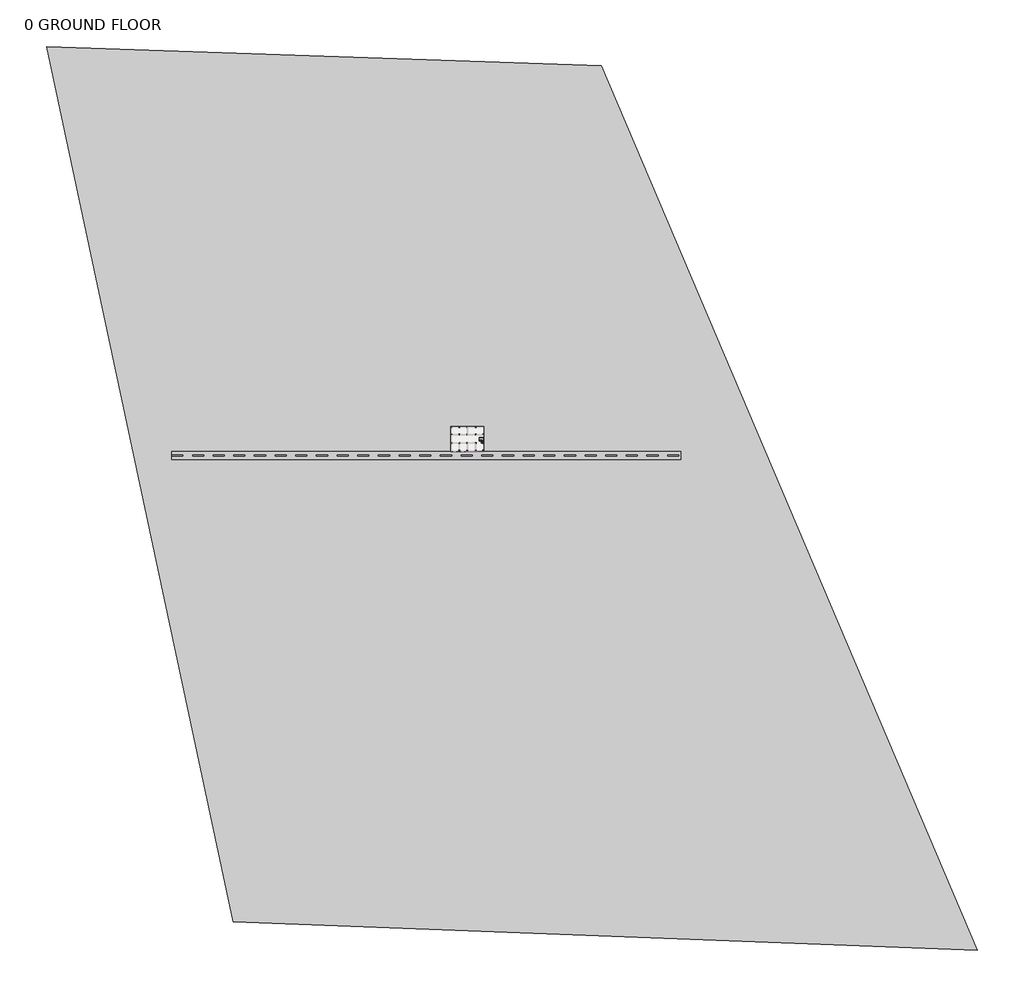
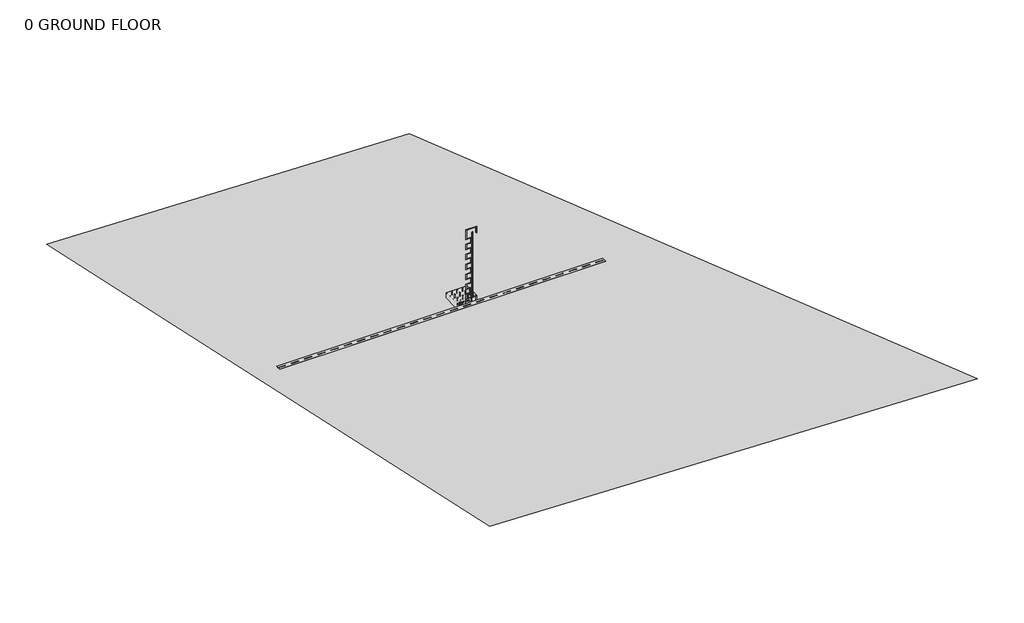
# One storey, part 2 of 2: 18 columns, 13 proxies, 4 members, 3 dampers, 2 cable carrier fittings, 1 stair flight.
"""IFC4 building model written with IfcOpenShell, lengths in millimetres."""

from ifc_helpers import new_model, si_unit, frame, origin, place, context, project, spatial, polyline, outline, extrude, faceted_brep, triangles, transform, mapped, element, save
from components import muntin_pattern_2x2_muntin_pattern_2x2_b3fe6957, muntin_pattern_2x2_muntin_pattern_2x2_3e0ecaf2, trim_window_exterior_flat_with_sill_41619996, trim_window_interior_flat_picture_frame_51c85655, conduit_fittings_1_conduit_fittings_1_d54f14cf, conduit_fittings_2_conduit_fittings_2_af195c82, duct_accessories_13_duct_accessories_1_4da7b8f5, duct_accessories_15_duct_accessories_15_503ec04a, duct_accessories_16_duct_accessories_15_820109d7, stair_flight_2b9b7e9b

model = new_model("IFC4")

# Units and contexts
model_context = context("Model", 3, world=origin())
ifc_project = project(units=[si_unit("LENGTHUNIT", "METRE", prefix="MILLI")], contexts=[model_context])

# Site, building, storey
site = spatial("IfcSite", under=ifc_project)
building = spatial("IfcBuilding", under=site)
storey = spatial("IfcBuildingStorey", under=building, Name="0 GROUND FLOOR", Elevation=0.0)

# Proxies
placement = place(None, origin())
element("IfcBuildingElementProxy", 1, Name="Building Element Proxy", at=placement, inside=storey, context=model_context, shape_type="Tessellation", body=[
    triangles([(-164952.4245117, 149002.5980713, 0.0), (39631.450708, 141833.0729004, 0.0), (178424.9416992, -184532.3270508, 0.0), (-96169.5159668, -174046.6042969, 0.0)], [[1, 4, 2], [3, 2, 4]], closed=False),
])
muntin_pattern_2x2_muntin_pattern_2x2_shape = muntin_pattern_2x2_muntin_pattern_2x2_b3fe6957(model_context)
element("IfcBuildingElementProxy", 2, Name="Muntin Pattern_2x2 : Muntin Pattern_2x2", ObjectType="Muntin Pattern_2x2 : Muntin Pattern_2x2", at=placement, inside=storey, context=model_context, shape_type="MappedRepresentation", body=[
    mapped(muntin_pattern_2x2_muntin_pattern_2x2_shape, transform((-14441.409625, -253.8184478, 984.25), x_axis=(1.0, 0.0, 0.0), y_axis=(0.0, 1.0, 0.0), z_axis=(0.0, 0.0, 1.0))),
])
element("IfcBuildingElementProxy", 3, Name="Muntin Pattern_2x2 : Muntin Pattern_2x2", ObjectType="Muntin Pattern_2x2 : Muntin Pattern_2x2", at=placement, inside=storey, context=model_context, shape_type="MappedRepresentation", body=[
    mapped(muntin_pattern_2x2_muntin_pattern_2x2_shape, transform((-11393.409625, -253.8184478, 984.25), x_axis=(1.0, 0.0, 0.0), y_axis=(0.0, 1.0, 0.0), z_axis=(0.0, 0.0, 1.0))),
])
element("IfcBuildingElementProxy", 4, Name="Muntin Pattern_2x2 : Muntin Pattern_2x2", ObjectType="Muntin Pattern_2x2 : Muntin Pattern_2x2", at=placement, inside=storey, context=model_context, shape_type="MappedRepresentation", body=[
    mapped(muntin_pattern_2x2_muntin_pattern_2x2_shape, transform((-8650.209625, -253.8184478, 984.25), x_axis=(1.0, 0.0, 0.0), y_axis=(0.0, 1.0, 0.0), z_axis=(0.0, 0.0, 1.0))),
])
muntin_pattern_2x2_muntin_pattern_2x2_2_shape = muntin_pattern_2x2_muntin_pattern_2x2_3e0ecaf2(model_context)
element("IfcBuildingElementProxy", 5, Name="Muntin Pattern_2x2 : Muntin Pattern_2x2", ObjectType="Muntin Pattern_2x2 : Muntin Pattern_2x2", at=placement, inside=storey, context=model_context, shape_type="MappedRepresentation", body=[
    mapped(muntin_pattern_2x2_muntin_pattern_2x2_2_shape, transform((-14012.784625, -253.8184478, 984.25), x_axis=(-1.0, 0.0, 0.0), y_axis=(0.0, -1.0, 0.0), z_axis=(0.0, 0.0, 1.0))),
])
element("IfcBuildingElementProxy", 6, Name="Muntin Pattern_2x2 : Muntin Pattern_2x2", ObjectType="Muntin Pattern_2x2 : Muntin Pattern_2x2", at=placement, inside=storey, context=model_context, shape_type="MappedRepresentation", body=[
    mapped(muntin_pattern_2x2_muntin_pattern_2x2_2_shape, transform((-10964.784625, -253.8184478, 984.25), x_axis=(-1.0, 0.0, 0.0), y_axis=(0.0, -1.0, 0.0), z_axis=(0.0, 0.0, 1.0))),
])
element("IfcBuildingElementProxy", 7, Name="Muntin Pattern_2x2 : Muntin Pattern_2x2", ObjectType="Muntin Pattern_2x2 : Muntin Pattern_2x2", at=placement, inside=storey, context=model_context, shape_type="MappedRepresentation", body=[
    mapped(muntin_pattern_2x2_muntin_pattern_2x2_2_shape, transform((-8221.584625, -253.8184478, 984.25), x_axis=(-1.0, 0.0, 0.0), y_axis=(0.0, -1.0, 0.0), z_axis=(0.0, 0.0, 1.0))),
])
trim_window_exterior_flat_with_sill_shape = trim_window_exterior_flat_with_sill_41619996(model_context)
element("IfcBuildingElementProxy", 8, Name="Trim-Window-Exterior-Flat : with Sill", ObjectType="Trim-Window-Exterior-Flat : with Sill", at=placement, inside=storey, context=model_context, shape_type="MappedRepresentation", body=[
    mapped(trim_window_exterior_flat_with_sill_shape, transform((-14227.097125, -244.2934478, 1828.8), x_axis=(-1.0, 0.0, 0.0), y_axis=(0.0, 0.0, 1.0), z_axis=(0.0, 1.0, 0.0))),
])
element("IfcBuildingElementProxy", 9, Name="Trim-Window-Exterior-Flat : with Sill", ObjectType="Trim-Window-Exterior-Flat : with Sill", at=placement, inside=storey, context=model_context, shape_type="MappedRepresentation", body=[
    mapped(trim_window_exterior_flat_with_sill_shape, transform((-11179.097125, -244.2934478, 1828.8), x_axis=(-1.0, 0.0, 0.0), y_axis=(0.0, 0.0, 1.0), z_axis=(0.0, 1.0, 0.0))),
])
element("IfcBuildingElementProxy", 10, Name="Trim-Window-Exterior-Flat : with Sill", ObjectType="Trim-Window-Exterior-Flat : with Sill", at=placement, inside=storey, context=model_context, shape_type="MappedRepresentation", body=[
    mapped(trim_window_exterior_flat_with_sill_shape, transform((-8435.897125, -244.2934478, 1828.8), x_axis=(-1.0, 0.0, 0.0), y_axis=(0.0, 0.0, 1.0), z_axis=(0.0, 1.0, 0.0))),
])
trim_window_interior_flat_picture_frame_shape = trim_window_interior_flat_picture_frame_51c85655(model_context)
element("IfcBuildingElementProxy", 11, Name="Trim-Window-Interior-Flat : Picture Frame", ObjectType="Trim-Window-Interior-Flat : Picture Frame", at=placement, inside=storey, context=model_context, shape_type="MappedRepresentation", body=[
    mapped(trim_window_interior_flat_picture_frame_shape, transform((-14227.097125, -371.2934478, 1828.8), x_axis=(1.0, 0.0, 0.0), y_axis=(0.0, 0.0, 1.0), z_axis=(0.0, -1.0, 0.0))),
])
element("IfcBuildingElementProxy", 12, Name="Trim-Window-Interior-Flat : Picture Frame", ObjectType="Trim-Window-Interior-Flat : Picture Frame", at=placement, inside=storey, context=model_context, shape_type="MappedRepresentation", body=[
    mapped(trim_window_interior_flat_picture_frame_shape, transform((-11179.097125, -371.2934478, 1828.8), x_axis=(1.0, 0.0, 0.0), y_axis=(0.0, 0.0, 1.0), z_axis=(0.0, -1.0, 0.0))),
])
element("IfcBuildingElementProxy", 13, Name="Trim-Window-Interior-Flat : Picture Frame", ObjectType="Trim-Window-Interior-Flat : Picture Frame", at=placement, inside=storey, context=model_context, shape_type="MappedRepresentation", body=[
    mapped(trim_window_interior_flat_picture_frame_shape, transform((-8435.897125, -371.2934478, 1828.8), x_axis=(1.0, 0.0, 0.0), y_axis=(0.0, 0.0, 1.0), z_axis=(0.0, -1.0, 0.0))),
])

# Cable carrier fittings
conduit_fittings_1_conduit_fittings_1_shape = conduit_fittings_1_conduit_fittings_1_d54f14cf(model_context)
element("IfcCableCarrierFitting", 14, ObjectType="Conduit Fittings 1 : Conduit Fittings 1", at=placement, inside=storey, context=model_context, shape_type="MappedRepresentation", body=[
    mapped(conduit_fittings_1_conduit_fittings_1_shape, transform((0.0, 0.0, 0.0), x_axis=(1.0, 0.0, 0.0), y_axis=(0.0, 1.0, 0.0), z_axis=(0.0, 0.0, 1.0))),
])
conduit_fittings_2_conduit_fittings_2_shape = conduit_fittings_2_conduit_fittings_2_af195c82(model_context)
element("IfcCableCarrierFitting", 15, ObjectType="Conduit Fittings 2 : Conduit Fittings 2", at=placement, inside=storey, context=model_context, shape_type="MappedRepresentation", body=[
    mapped(conduit_fittings_2_conduit_fittings_2_shape, transform((0.0, 0.0, 0.0), x_axis=(1.0, 0.0, 0.0), y_axis=(0.0, 1.0, 0.0), z_axis=(0.0, 0.0, 1.0))),
])

# Columns
element("IfcColumn", 16, ObjectType="column family : column family", at=placement, inside=storey, context=model_context, shape_type="SweptSolid", body=[
    extrude(outline(polyline([(-15433.597125, 8645.7065522), (-15433.597125, 8391.7065522), (-15687.597125, 8391.7065522), (-15687.597125, 8645.7065522), (-15433.597125, 8645.7065522)])), frame((0.0, 0.0, 5.0), z_axis=(0.0, 0.0, 1.0), x_axis=(1.0, 0.0, 0.0)), (0.0, 0.0, 1.0), 3038.0),
])
element("IfcColumn", 17, ObjectType="column family : column family", at=placement, inside=storey, context=model_context, shape_type="SweptSolid", body=[
    extrude(outline(polyline([(-12576.097125, 5915.2065522), (-12576.097125, 5534.2065522), (-12957.097125, 5534.2065522), (-12957.097125, 5915.2065522), (-12576.097125, 5915.2065522)])), frame((0.0, 0.0, 5.0), z_axis=(0.0, 0.0, 1.0), x_axis=(1.0, 0.0, 0.0)), (0.0, 0.0, 1.0), 3038.0),
])
element("IfcColumn", 18, ObjectType="column family : column family", at=placement, inside=storey, context=model_context, shape_type="Brep", body=[
    faceted_brep([(-9655.097125, 5915.2065522, 5.0), (-9528.097125, 5915.2065522, 5.0), (-9528.097125, 5788.2065522, 5.0), (-9655.097125, 5788.2065522, 5.0), (-9528.097125, 5915.2065522, 3043.0), (-9655.097125, 5915.2065522, 3043.0), (-9655.097125, 5788.2065522, 3043.0), (-9528.097125, 5788.2065522, 3043.0)], [[[0, 1, 2, 3]], [[4, 5, 6, 7]], [[0, 3, 6, 5]], [[4, 1, 0, 5]], [[3, 2, 7, 6]], [[1, 4, 7, 2]]]),
    faceted_brep([(-9528.097125, 5534.2065522, 3043.0), (-9528.097125, 5534.2065522, 5.0), (-9528.097125, 5661.2065522, 5.0), (-9528.097125, 5661.2065522, 3043.0), (-9909.097125, 5534.2065522, 5.0), (-9909.097125, 5534.2065522, 3043.0), (-9909.097125, 5915.2065522, 5.0), (-9909.097125, 5661.2065522, 3043.0), (-9909.097125, 5661.2065522, 2133.6), (-9909.097125, 5788.2065522, 2133.6), (-9909.097125, 5788.2065522, 3043.0), (-9909.097125, 5915.2065522, 3043.0), (-9782.097125, 5915.2065522, 3043.0), (-9782.097125, 5915.2065522, 5.0), (-9782.097125, 5788.2065522, 5.0), (-9782.097125, 5788.2065522, 3043.0), (-9782.097125, 5788.2065522, 2133.6), (-9718.597125, 5788.2065522, 5.0), (-9718.597125, 5788.2065522, 2133.6), (-9718.597125, 5661.2065522, 5.0), (-9718.597125, 5661.2065522, 2133.6)], [[[0, 1, 2, 3]], [[4, 1, 0, 5]], [[6, 4, 5, 7, 8, 9, 10, 11]], [[6, 11, 12, 13]], [[14, 13, 12, 15, 16]], [[17, 14, 16, 18]], [[19, 20, 8, 7, 3, 2]], [[1, 4, 6, 13, 14, 17, 19, 2]], [[5, 0, 3, 7]], [[12, 11, 10, 15]], [[9, 16, 15, 10]], [[18, 20, 19, 17]], [[20, 18, 16, 9, 8]]]),
])
element("IfcColumn", 19, ObjectType="column family : column family", at=placement, inside=storey, context=model_context, shape_type="Brep", body=[
    faceted_brep([(-6480.097125, 5534.2065522, 5.0), (-6861.097125, 5534.2065522, 5.0), (-6861.097125, 5915.2065522, 5.0), (-6480.097125, 5915.2065522, 5.0), (-6480.097125, 5788.2065522, 5.0), (-6670.597125, 5788.2065522, 5.0), (-6670.597125, 5661.2065522, 5.0), (-6480.097125, 5661.2065522, 5.0), (-6480.097125, 5534.2065522, 3043.0), (-6480.097125, 5661.2065522, 3043.0), (-6861.097125, 5534.2065522, 3043.0), (-6861.097125, 5661.2065522, 3043.0), (-6861.097125, 5661.2065522, 2133.6), (-6861.097125, 5788.2065522, 2133.6), (-6861.097125, 5788.2065522, 3043.0), (-6861.097125, 5915.2065522, 3043.0), (-6480.097125, 5915.2065522, 3043.0), (-6670.597125, 5661.2065522, 2133.6), (-6670.597125, 5788.2065522, 2133.6), (-6480.097125, 5788.2065522, 3043.0)], [[[0, 1, 2, 3, 4, 5, 6, 7]], [[8, 0, 7, 9]], [[1, 0, 8, 10]], [[2, 1, 10, 11, 12, 13, 14, 15]], [[3, 2, 15, 16]], [[10, 8, 9, 11]], [[6, 17, 12, 11, 9, 7]], [[13, 18, 5, 4, 19, 14]], [[3, 16, 19, 4]], [[16, 15, 14, 19]], [[18, 17, 6, 5]], [[17, 18, 13, 12]]]),
])
element("IfcColumn", 20, ObjectType="column family : column family", at=placement, inside=storey, context=model_context, shape_type="Brep", body=[
    faceted_brep([(-6480.097125, 2867.2065522, 5.0), (-6480.097125, 2486.2065522, 5.0), (-6645.197125, 2486.2065522, 5.0), (-6645.197125, 2740.2065522, 5.0), (-6708.697125, 2740.2065522, 5.0), (-6708.697125, 2613.2065522, 5.0), (-6772.197125, 2613.2065522, 5.0), (-6772.197125, 2486.2065522, 5.0), (-6861.097125, 2486.2065522, 5.0), (-6861.097125, 2867.2065522, 5.0), (-6480.097125, 2867.2065522, 3043.0), (-6480.097125, 2486.2065522, 3043.0), (-6861.097125, 2486.2065522, 3043.0), (-6772.197125, 2486.2065522, 3043.0), (-6861.097125, 2613.2065522, 3043.0), (-6861.097125, 2613.2065522, 2133.6), (-6861.097125, 2740.2065522, 2133.6), (-6861.097125, 2740.2065522, 3043.0), (-6861.097125, 2867.2065522, 3043.0), (-6772.197125, 2740.2065522, 3043.0), (-6645.197125, 2740.2065522, 3043.0), (-6645.197125, 2486.2065522, 3043.0), (-6772.197125, 2613.2065522, 3043.0), (-6772.197125, 2613.2065522, 2133.6), (-6772.197125, 2740.2065522, 2133.6), (-6708.697125, 2613.2065522, 2133.6), (-6708.697125, 2740.2065522, 2133.6)], [[[0, 1, 2, 3, 4, 5, 6, 7, 8, 9]], [[1, 0, 10, 11]], [[12, 8, 7, 13]], [[9, 8, 12, 14, 15, 16, 17, 18]], [[0, 9, 18, 10]], [[11, 10, 18, 17, 19, 20, 21]], [[15, 14, 22, 23]], [[17, 16, 24, 19]], [[20, 3, 2, 21]], [[6, 23, 22, 13, 7]], [[14, 12, 13, 22]], [[1, 11, 21, 2]], [[15, 23, 24, 16]], [[25, 23, 6, 5]], [[23, 25, 26, 24]], [[26, 25, 5, 4]], [[24, 26, 4, 3, 20, 19]]]),
])
element("IfcColumn", 21, ObjectType="column family : column family", at=placement, inside=storey, context=model_context, shape_type="Brep", body=[
    faceted_brep([(-9528.097125, 2486.2065522, 5.0), (-9909.097125, 2486.2065522, 5.0), (-9909.097125, 2867.2065522, 5.0), (-9528.097125, 2867.2065522, 5.0), (-9528.097125, 2740.2065522, 5.0), (-9566.197125, 2740.2065522, 5.0), (-9718.597125, 2740.2065522, 5.0), (-9718.597125, 2613.2065522, 5.0), (-9566.197125, 2613.2065522, 5.0), (-9528.097125, 2613.2065522, 5.0), (-9528.097125, 2486.2065522, 3043.0), (-9528.097125, 2613.2065522, 304.8), (-9528.097125, 2740.2065522, 304.8), (-9528.097125, 2867.2065522, 3043.0), (-9528.097125, 2740.2065522, 3043.0), (-9528.097125, 2740.2065522, 2133.6), (-9528.097125, 2613.2065522, 2133.6), (-9528.097125, 2613.2065522, 3043.0), (-9909.097125, 2486.2065522, 3043.0), (-9909.097125, 2867.2065522, 3043.0), (-9566.197125, 2613.2065522, 3043.0), (-9718.597125, 2613.2065522, 3043.0), (-9718.597125, 2740.2065522, 3043.0), (-9566.197125, 2740.2065522, 3043.0), (-9566.197125, 2613.2065522, 2133.6), (-9566.197125, 2613.2065522, 304.8), (-9566.197125, 2740.2065522, 304.8), (-9566.197125, 2740.2065522, 2133.6)], [[[0, 1, 2, 3, 4, 5, 6, 7, 8, 9]], [[10, 0, 9, 11, 12, 4, 3, 13, 14, 15, 16, 17]], [[1, 0, 10, 18]], [[2, 1, 18, 19]], [[3, 2, 19, 13]], [[18, 10, 17, 20, 21, 22, 23, 14, 13, 19]], [[11, 9, 8, 7, 21, 20, 17, 16, 24, 25]], [[4, 12, 26, 27, 15, 14, 23, 22, 6, 5]], [[21, 7, 6, 22]], [[25, 24, 27, 26]], [[25, 26, 12, 11]], [[27, 24, 16, 15]]]),
])
element("IfcColumn", 22, ObjectType="column family : column family", at=placement, inside=storey, context=model_context, shape_type="Brep", body=[
    faceted_brep([(-12576.097125, 2486.2065522, 5.0), (-12957.097125, 2486.2065522, 5.0), (-12957.097125, 2867.2065522, 5.0), (-12576.097125, 2867.2065522, 5.0), (-12576.097125, 2740.2065522, 5.0), (-12842.797125, 2740.2065522, 5.0), (-12842.797125, 2613.2065522, 5.0), (-12576.097125, 2613.2065522, 5.0), (-12576.097125, 2486.2065522, 3043.0), (-12576.097125, 2613.2065522, 3043.0), (-12957.097125, 2486.2065522, 3043.0), (-12957.097125, 2613.2065522, 3043.0), (-12957.097125, 2613.2065522, 2133.6), (-12957.097125, 2740.2065522, 2133.6), (-12957.097125, 2740.2065522, 3043.0), (-12957.097125, 2867.2065522, 3043.0), (-12576.097125, 2867.2065522, 3043.0), (-12842.797125, 2613.2065522, 2133.6), (-12842.797125, 2740.2065522, 2133.6), (-12576.097125, 2740.2065522, 3043.0)], [[[0, 1, 2, 3, 4, 5, 6, 7]], [[8, 0, 7, 9]], [[1, 0, 8, 10]], [[2, 1, 10, 11, 12, 13, 14, 15]], [[3, 2, 15, 16]], [[10, 8, 9, 11]], [[6, 17, 12, 11, 9, 7]], [[13, 18, 5, 4, 19, 14]], [[3, 16, 19, 4]], [[16, 15, 14, 19]], [[17, 18, 13, 12]], [[18, 17, 6, 5]]]),
])
element("IfcColumn", 23, ObjectType="column family : column family", at=placement, inside=storey, context=model_context, shape_type="SweptSolid", body=[
    extrude(outline(polyline([(-12576.097125, 8391.7065522), (-12957.097125, 8391.7065522), (-12957.097125, 8645.7065522), (-12576.097125, 8645.7065522), (-12576.097125, 8391.7065522)])), frame((0.0, 0.0, 5.0), z_axis=(0.0, 0.0, 1.0), x_axis=(1.0, 0.0, 0.0)), (0.0, 0.0, 1.0), 3038.0),
])
element("IfcColumn", 24, ObjectType="column family : column family", at=placement, inside=storey, context=model_context, shape_type="SweptSolid", body=[
    extrude(outline(polyline([(-9528.097125, 8391.7065522), (-9909.097125, 8391.7065522), (-9909.097125, 8645.7065522), (-9528.097125, 8645.7065522), (-9528.097125, 8391.7065522)])), frame((0.0, 0.0, 5.0), z_axis=(0.0, 0.0, 1.0), x_axis=(1.0, 0.0, 0.0)), (0.0, 0.0, 1.0), 3038.0),
])
element("IfcColumn", 25, ObjectType="column family : column family", at=placement, inside=storey, context=model_context, shape_type="SweptSolid", body=[
    extrude(outline(polyline([(-6480.097125, 8391.7065522), (-6861.097125, 8391.7065522), (-6861.097125, 8645.7065522), (-6480.097125, 8645.7065522), (-6480.097125, 8391.7065522)])), frame((0.0, 0.0, 5.0), z_axis=(0.0, 0.0, 1.0), x_axis=(1.0, 0.0, 0.0)), (0.0, 0.0, 1.0), 3038.0),
])
element("IfcColumn", 26, ObjectType="column family : column family", at=placement, inside=storey, context=model_context, shape_type="SweptSolid", body=[
    extrude(outline(polyline([(-4003.597125, 5915.2065522), (-3749.597125, 5915.2065522), (-3749.597125, 5788.2065522), (-4003.597125, 5788.2065522), (-4003.597125, 5915.2065522)])), frame((0.0, 0.0, 5.0), z_axis=(0.0, 0.0, 1.0), x_axis=(1.0, 0.0, 0.0)), (0.0, 0.0, 1.0), 3038.0),
    extrude(outline(polyline([(-3749.597125, 5534.2065522), (-4003.597125, 5534.2065522), (-4003.597125, 5661.2065522), (-3749.597125, 5661.2065522), (-3749.597125, 5534.2065522)])), frame((0.0, 0.0, 5.0), z_axis=(0.0, 0.0, 1.0), x_axis=(1.0, 0.0, 0.0)), (0.0, 0.0, 1.0), 3038.0),
])
element("IfcColumn", 27, ObjectType="column family : column family", at=placement, inside=storey, context=model_context, shape_type="SweptSolid", body=[
    extrude(outline(polyline([(-4003.597125, 2486.2065522), (-4003.597125, 2867.2065522), (-3749.597125, 2867.2065522), (-3749.597125, 2486.2065522), (-4003.597125, 2486.2065522)])), frame((0.0, 0.0, 5.0), z_axis=(0.0, 0.0, 1.0), x_axis=(1.0, 0.0, 0.0)), (0.0, 0.0, 1.0), 3038.0),
])
element("IfcColumn", 28, ObjectType="column family : column family", at=placement, inside=storey, context=model_context, shape_type="SweptSolid", body=[
    extrude(outline(polyline([(-15433.597125, 5915.2065522), (-15433.597125, 5534.2065522), (-15687.597125, 5534.2065522), (-15687.597125, 5915.2065522), (-15433.597125, 5915.2065522)])), frame((0.0, 0.0, 5.0), z_axis=(0.0, 0.0, 1.0), x_axis=(1.0, 0.0, 0.0)), (0.0, 0.0, 1.0), 3038.0),
])
element("IfcColumn", 29, ObjectType="column family : column family", at=placement, inside=storey, context=model_context, shape_type="SweptSolid", body=[
    extrude(outline(polyline([(-15433.597125, 2867.2065522), (-15433.597125, 2486.2065522), (-15687.597125, 2486.2065522), (-15687.597125, 2867.2065522), (-15433.597125, 2867.2065522)])), frame((0.0, 0.0, 5.0), z_axis=(0.0, 0.0, 1.0), x_axis=(1.0, 0.0, 0.0)), (0.0, 0.0, 1.0), 3038.0),
])
element("IfcColumn", 30, ObjectType="column family : column family", at=placement, inside=storey, context=model_context, shape_type="SweptSolid", body=[
    extrude(outline(polyline([(-3622.597125, -371.2934478), (-4003.597125, -371.2934478), (-4003.597125, 9.7065522), (-3749.597125, 9.7065522), (-3749.597125, -307.7934478), (-3622.597125, -307.7934478), (-3622.597125, -371.2934478)])), frame((0.0, 0.0, 5.0), z_axis=(0.0, 0.0, 1.0), x_axis=(1.0, 0.0, 0.0)), (0.0, 0.0, 1.0), 3038.0),
])
element("IfcColumn", 31, ObjectType="column family : column family", at=placement, inside=storey, context=model_context, shape_type="SweptSolid", body=[
    extrude(outline(polyline([(-6480.097125, 9.7065522), (-6480.097125, -371.2934478), (-6861.097125, -371.2934478), (-6861.097125, 9.7065522), (-6480.097125, 9.7065522)])), frame((0.0, 0.0, 5.0), z_axis=(0.0, 0.0, 1.0), x_axis=(1.0, 0.0, 0.0)), (0.0, 0.0, 1.0), 3038.0),
])
element("IfcColumn", 32, ObjectType="column family : column family", at=placement, inside=storey, context=model_context, shape_type="SweptSolid", body=[
    extrude(outline(polyline([(-9909.097125, 9.7065522), (-9528.097125, 9.7065522), (-9528.097125, -244.2934478), (-9909.097125, -244.2934478), (-9909.097125, 9.7065522)])), frame((0.0, 0.0, 5.0), z_axis=(0.0, 0.0, 1.0), x_axis=(1.0, 0.0, 0.0)), (0.0, 0.0, 1.0), 3038.0),
])
element("IfcColumn", 33, ObjectType="column family : column family", at=placement, inside=storey, context=model_context, shape_type="SweptSolid", body=[
    extrude(outline(polyline([(-12957.097125, 9.7065522), (-12576.097125, 9.7065522), (-12576.097125, -244.2934478), (-12957.097125, -244.2934478), (-12957.097125, 9.7065522)])), frame((0.0, 0.0, 5.0), z_axis=(0.0, 0.0, 1.0), x_axis=(1.0, 0.0, 0.0)), (0.0, 0.0, 1.0), 3038.0),
])

# Dampers
duct_accessories_13_duct_accessories_1_shape = duct_accessories_13_duct_accessories_1_4da7b8f5(model_context)
element("IfcDamper", 34, ObjectType="Duct Accessories 13 : Duct Accessories 1", at=placement, inside=storey, context=model_context, shape_type="MappedRepresentation", body=[
    mapped(duct_accessories_13_duct_accessories_1_shape, transform((0.0, 0.0, 0.0), x_axis=(1.0, 0.0, 0.0), y_axis=(0.0, 1.0, 0.0), z_axis=(0.0, 0.0, 1.0))),
])
duct_accessories_15_duct_accessories_15_shape = duct_accessories_15_duct_accessories_15_503ec04a(model_context)
element("IfcDamper", 35, ObjectType="Duct Accessories 15 : Duct Accessories 15", at=placement, inside=storey, context=model_context, shape_type="MappedRepresentation", body=[
    mapped(duct_accessories_15_duct_accessories_15_shape, transform((0.0, 0.0, 0.0), x_axis=(1.0, 0.0, 0.0), y_axis=(0.0, 1.0, 0.0), z_axis=(0.0, 0.0, 1.0))),
])
duct_accessories_16_duct_accessories_15_shape = duct_accessories_16_duct_accessories_15_820109d7(model_context)
element("IfcDamper", 36, ObjectType="Duct Accessories 16 : Duct Accessories 15", at=placement, inside=storey, context=model_context, shape_type="MappedRepresentation", body=[
    mapped(duct_accessories_16_duct_accessories_15_shape, transform((0.0, 0.0, 0.0), x_axis=(1.0, 0.0, 0.0), y_axis=(0.0, 1.0, 0.0), z_axis=(0.0, 0.0, 1.0))),
])

# Members
element("IfcMember", 37, ObjectType="Stringer - 2\" Width", at=placement, inside=storey, context=model_context, shape_type="SweptSolid", body=[
    extrude(outline(polyline([(2714.6319226, 0.0), (2714.6319226, 236.8438745), (3679.8319226, 1041.1772078), (3679.8319226, 644.4165243), (2906.5320935, 0.0), (2714.6319226, 0.0)])), frame((-4563.0136682, 0.0, 0.0), z_axis=(1.0, 0.0, 0.0), x_axis=(0.0, 1.0, 0.0)), (0.0, 0.0, 1.0), 50.8),
])
element("IfcMember", 38, ObjectType="Stringer - 2\" Width", at=placement, inside=storey, context=model_context, shape_type="SweptSolid", body=[
    extrude(outline(polyline([(-4512.2136682, 3730.6319226), (-4512.2136682, 3679.8319226), (-4563.0136682, 3679.8319226), (-4563.0136682, 3730.6319226), (-4512.2136682, 3730.6319226)])), frame((0.0, 0.0, 787.4), z_axis=(0.0, 0.0, 1.0), x_axis=(1.0, 0.0, 0.0)), (0.0, 0.0, 1.0), 304.8),
])
element("IfcMember", 39, ObjectType="Stringer - 2\" Width", at=placement, inside=storey, context=model_context, shape_type="SweptSolid", body=[
    extrude(outline(polyline([(2714.6319226, 0.0), (2714.6319226, 236.8438745), (3741.0592732, 1092.2), (4217.1720935, 1092.2), (2906.5320935, 0.0), (2714.6319226, 0.0)])), frame((-3749.597125, 0.0, 0.0), z_axis=(1.0, 0.0, 0.0), x_axis=(0.0, 1.0, 0.0)), (0.0, 0.0, 1.0), 50.8),
])
element("IfcMember", 40, ObjectType="Stringer - 2\" Width", at=placement, inside=storey, context=model_context, shape_type="SweptSolid", body=[
    extrude(outline(polyline([(-3698.797125, 4695.8319226), (-3698.797125, 4645.0319226), (-5295.0246464, 4645.0319226), (-5295.0246464, 4695.8319226), (-3698.797125, 4695.8319226)])), frame((0.0, 0.0, 787.4), z_axis=(0.0, 0.0, 1.0), x_axis=(1.0, 0.0, 0.0)), (0.0, 0.0, 1.0), 304.8),
])

# Stair flight
stair_flight_shape = stair_flight_2b9b7e9b(model_context)
element("IfcStairFlight", 41, ObjectType="2\" Tread 1\" Nosing 1/4\" Riser", at=placement, inside=storey, context=model_context, shape_type="MappedRepresentation", body=[
    mapped(stair_flight_shape, transform((0.0, 0.0, 0.0), x_axis=(1.0, 0.0, 0.0), y_axis=(0.0, 1.0, 0.0), z_axis=(0.0, 0.0, 1.0))),
])

save(model, "model.ifc")

# Revit data of these elements
# Type "Muntin Pattern_2x2 : Muntin Pattern_2x2"
#   Width [instance default] = 4' - 0"
#   Thickness = 0' - 0 1/2"
#   Height [instance default] = 4' - 0"
#   Distance = 0' - 0 3/4"
#   Interior Material [instance default] = none
#   Exterior Material [instance default] = none
#   Default Elevation = 0
# Type "Trim-Window-Exterior-Flat : with Sill"
#   Trim Width = 0' - 2 1/4"
#   Trim Thickness_Picture Frame = 0' - 1 1/4"
#   Trim Thickness_with Sill = 0' - 0 3/4"
#   Sill Thickness = 0' - 1 1/4"
#   Opening Width [instance default] = 2' - 0"
#   Opening Height [instance default] = 3' - 0"
#   Default Elevation = 4' - 0"
#   Sill = yes
#   Picture Frame = no
#   Trim Material [instance default] = none
# Type "Trim-Window-Interior-Flat : Picture Frame"
#   Trim Thickness_Picture Frame = 0' - 1 1/4"
#   Trim Width = 0' - 2 1/4"
#   Trim Thickness_with Sill = 0' - 0 3/4"
#   Sill Thickness = 0' - 1 1/4"
#   Opening Width [instance default] = 2' - 0"
#   Opening Height [instance default] = 3' - 0"
#   Default Elevation = 4' - 0"
#   Sill = no
#   Picture Frame = yes
#   Trim Material [instance default] = none
# Type "column family : column family"
#   w2 [instance default] = 0' - 9.88189"
#   w1 [instance default] = 0' - 9.01575"
#   Depth = 1' - 11.62205"
#   Width = 1' - 11.62205"
# Element 1 (IfcBuildingElementProxy)
#   Material = gras
#   Phase Created = New Construction
# Elements 2, 3, 4, 5, 6, 7 (IfcBuildingElementProxy, "Muntin Pattern_2x2 : Muntin Pattern_2x2")
#   Width = 0' - 11 5/8"
#   Height = 2' - 6 1/2"
#   Interior Material = Wood - Stained
#   Exterior Material = Clad - White
#   Phase Created = New Construction
#   Materials on its faces: "Clad - White", "Wood - Stained"
# Elements 8, 9, 10 (IfcBuildingElementProxy, "Trim-Window-Exterior-Flat : with Sill")
#   Opening Width = 2' - 10"
#   Opening Height = 3' - 0"
#   Trim Material = Clad - White
#   Phase Created = New Construction
#   Materials on its faces: "Clad - White"
# Elements 11, 12, 13 (IfcBuildingElementProxy, "Trim-Window-Interior-Flat : Picture Frame")
#   Opening Width = 2' - 10"
#   Opening Height = 3' - 0"
#   Trim Material = Wood - Stained
#   Phase Created = New Construction
#   Materials on its faces: "Wood - Stained"
# Element 14 (IfcCableCarrierFitting, "Conduit Fittings 1 : Conduit Fittings 1")
#   built-in parameter 1140129 = 2
#   Phase Created = New Construction
#   Materials on its faces: "yellow"
# Element 15 (IfcCableCarrierFitting, "Conduit Fittings 2 : Conduit Fittings 2")
#   built-in parameter 1140129 = 2
#   Phase Created = New Construction
# Elements 16, 17, 18, 23, 24, 25, 32, 33 (IfcColumn, "column family : column family")
#   w2 = 1' - 3"
#   w1 = 1' - 3"
#   Phase Created = New Construction
#   Materials on its faces: "Default Wall"
# Elements 19, 26, 27 (IfcColumn, "column family : column family")
#   w2 = 1' - 3"
#   w1 = 1' - 3"
#   Phase Created = New Construction
#   Materials on its faces: "grey", "Default Wall"
# Element 20 (IfcColumn, "column family : column family")
#   w2 = 1' - 3"
#   w1 = 1' - 3"
#   Phase Created = New Construction
#   Materials on its faces: "Default Wall", "grey"
# Elements 21, 22 (IfcColumn, "column family : column family")
#   w2 = 1' - 3"
#   w1 = 1' - 3"
#   Phase Created = New Construction
#   Materials on its faces: "Default Wall", "inside wall"
# Element 28 (IfcColumn, "column family : column family")
#   w2 = 1' - 3"
#   w1 = 1' - 3"
#   Phase Created = New Construction
#   Materials on its faces: "inside wall", "Default Wall"
# Element 29 (IfcColumn, "column family : column family")
#   w2 = 1' - 3"
#   w1 = 0' - 10"
#   Phase Created = New Construction
#   Materials on its faces: "inside wall", "Default Wall"
# Element 30 (IfcColumn, "column family : column family")
#   w2 = 1' - 3"
#   w1 = 1' - 3"
#   Phase Created = New Construction
#   Materials on its faces: "grey", "Default Wall", "Clad - White"
# Element 31 (IfcColumn, "column family : column family")
#   w2 = 1' - 3"
#   w1 = 1' - 3"
#   Phase Created = New Construction
#   Materials on its faces: "out side wall", "Default Wall"
# Element 34 (IfcDamper, "Duct Accessories 13 : Duct Accessories 1")
#   Mark = "13"
#   Phase Created = New Construction
#   Materials on its faces: "border"
# Element 35 (IfcDamper, "Duct Accessories 15 : Duct Accessories 15")
#   Mark = "15"
#   Phase Created = New Construction
#   Materials on its faces: "road"
# Element 36 (IfcDamper, "Duct Accessories 16 : Duct Accessories 15")
#   Mark = "16"
#   Phase Created = New Construction
#   Materials on its faces: "Clad - White"
# Elements 37, 38, 39, 40 (IfcMember, "Stringer - 2\" Width")
#   Phase Created = New Construction
# Element 41 (IfcStairFlight, "2\" Tread 1\" Nosing 1/4\" Riser")
#   Phase Created = New Construction
# Materials
#   "gras": class "Generic", colour RGB 40 117 68, transparency 0, Cost = 0
#   "Clad - White": class "Wood", colour RGB 242 242 238, transparency 0, Cost = 0
#   "Wood - Stained": class "Wood", colour RGB 224 178 126, transparency 0, Cost = 0
#   "yellow": class "Generic", colour RGB 255 255 0, transparency 0, Cost = 0
#   "Default Wall": colour RGB 128 128 128, transparency 0, Cost = 0
#   "grey": class "Generic", colour RGB 80 80 80, transparency 0, Cost = 0
#   "inside wall": class "Generic", colour RGB 199 224 95, transparency 0, Cost = 0
#   "out side wall": class "Generic", colour RGB 16 106 159, transparency 0, Cost = 0
#   "border": class "Generic", colour RGB 144 144 144, transparency 0, Cost = 0
#   "road": class "Generic", colour RGB 0 0 0, transparency 0, Cost = 0
